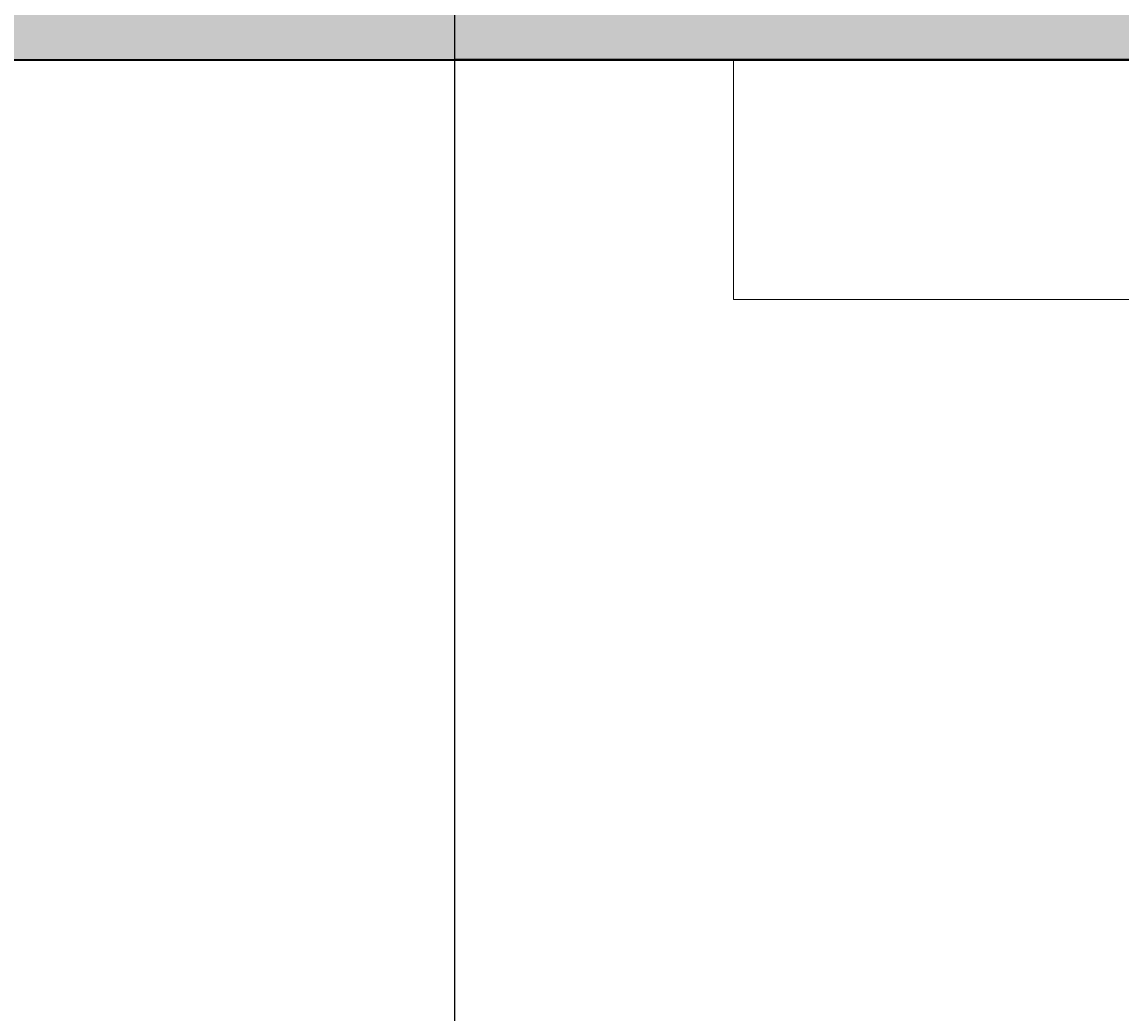
# Model space of a CAD drawing. Units: inches. Extents: x 1998 to 2588, y 1139 to 1977.
# Tile 84 of 134: x 2397 to 2425, y 1452 to 1477. Entities that reach past the tile are written whole.
import ezdxf

# ---------------------------------------------------------------- set-up
doc = ezdxf.new("R2010")
doc.units = ezdxf.units.IN
for name, color, linetype, lineweight in [('A-ANNO-DIMS', 2, 'Continuous', 18), ('A-WALL-PATT', 252, 'Continuous', 13), ('FUR', 21, 'Continuous', 18), ('WALL', 200, 'Continuous', 35)]:
    doc.layers.add(name, color=color, linetype=linetype, lineweight=lineweight)
doc.styles.get("Standard").update_dxf_attribs({"font": 'arial.ttf'})
doc.dimstyles.get("Standard").update_dxf_attribs({"dimtxt": 0.18, "dimasz": 0.18, "dimexe": 0.18, "dimexo": 0.0625, "dimgap": 0.09, "dimtad": 0, "dimtih": 1, "dimtoh": 1, "dimdec": 4, "dimzin": 0, "dimdsep": 46, "dimtxsty": 'Standard', "dimcen": 0.09, "dimadec": 0, "dimazin": 0, "dimtfac": 1, "dimtdec": 4, "dimtofl": 0, "dimtmove": 0, "dimatfit": 3, "dimfxl": 1, "dimtolj": 1, "dimtzin": 0, "dimarcsym": 0})

# ---------------------------------------------------------------- blocks, each defined once
blk = doc.blocks.new('CONSOLE-WALL')
blk.add_lwpolyline([(0, 6.123), (71.98, 6.123), (71.98, 0), (0, 0)], close=True)
blk = doc.blocks.new('*D23')
at = {"layer": 'A-ANNO-DIMS', "color": 0, "lineweight": -2, "transparency": 16777216}
for p, q in [((2549.179, 1476.17), (2549.179, 1138.602)), ((2059.473, 1413.17), (2059.473, 1138.602)), ((2059.653, 1138.782), (2303.928, 1138.782)), ((2548.999, 1138.782), (2304.723, 1138.782))]:
    blk.add_line(p, q, dxfattribs=at)
at = {"layer": 'A-ANNO-DIMS', "color": 0, "transparency": 16777216}
for points in [[(2059.653, 1138.812), (2059.653, 1138.752), (2059.473, 1138.782)], [(2548.999, 1138.812), (2548.999, 1138.752), (2549.179, 1138.782)]]:
    blk.add_solid(points, dxfattribs=at)
at = {"layer": 'Defpoints', "color": 0, "transparency": 16777216}
for p in [(2549.179, 1476.232), (2059.473, 1413.232), (2549.179, 1138.782)]:
    blk.add_point(p, dxfattribs=at)
at = {"layer": 'A-ANNO-DIMS', "color": 0, "transparency": 16777216, "insert": (2304.326, 1138.782), "char_height": 0.18, "attachment_point": 5}
blk.add_mtext('\\A1;489.7', dxfattribs=at)
blk = doc.blocks.new('*D24')
at = {"layer": 'A-ANNO-DIMS', "color": 0, "lineweight": -2, "transparency": 16777216}
for p, q in [((2398.535, 1911.232), (2588.309, 1911.232)), ((2588.129, 1911.052), (2588.129, 1570.164)), ((2588.129, 1228.912), (2588.129, 1569.8)), ((2527.535, 1228.732), (2588.309, 1228.732))]:
    blk.add_line(p, q, dxfattribs=at)
at = {"layer": 'A-ANNO-DIMS', "color": 0, "transparency": 16777216}
for points in [[(2588.099, 1911.052), (2588.159, 1911.052), (2588.129, 1911.232)], [(2588.099, 1228.912), (2588.159, 1228.912), (2588.129, 1228.732)]]:
    blk.add_solid(points, dxfattribs=at)
at = {"layer": 'Defpoints', "color": 0, "transparency": 16777216}
for p in [(2398.473, 1911.232), (2588.129, 1911.232), (2527.473, 1228.732)]:
    blk.add_point(p, dxfattribs=at)
at = {"layer": 'A-ANNO-DIMS', "color": 0, "transparency": 16777216, "insert": (2588.129, 1569.982), "char_height": 0.18, "attachment_point": 5}
blk.add_mtext('\\A1;682.5', dxfattribs=at)
blk = doc.blocks.new('*D33')
at = {"layer": 'A-ANNO-DIMS', "color": 0, "lineweight": -2, "transparency": 16777216}
for p, q in [((2407.973, 1480.67), (2407.973, 1138.602)), ((2498.179, 1480.67), (2498.179, 1138.602)), ((2408.153, 1138.782), (2452.753, 1138.782)), ((2497.999, 1138.782), (2453.399, 1138.782))]:
    blk.add_line(p, q, dxfattribs=at)
at = {"layer": 'A-ANNO-DIMS', "color": 0, "transparency": 16777216}
for points in [[(2408.153, 1138.812), (2408.153, 1138.752), (2407.973, 1138.782)], [(2497.999, 1138.812), (2497.999, 1138.752), (2498.179, 1138.782)]]:
    blk.add_solid(points, dxfattribs=at)
at = {"layer": 'Defpoints', "color": 0, "transparency": 16777216}
for p in [(2407.973, 1480.732), (2498.179, 1480.732), (2498.179, 1138.782)]:
    blk.add_point(p, dxfattribs=at)
at = {"layer": 'A-ANNO-DIMS', "color": 0, "transparency": 16777216, "insert": (2453.076, 1138.782), "char_height": 0.18, "attachment_point": 5}
blk.add_mtext('\\A1;90.2', dxfattribs=at)
blk = doc.blocks.new('*D43')
at = {"layer": 'A-ANNO-DIMS', "color": 0, "lineweight": -2, "transparency": 16777216}
for p, q in [((2407.973, 1594.67), (2407.973, 1138.602)), ((2345.973, 1588.67), (2345.973, 1138.602)), ((2346.153, 1138.782), (2376.754, 1138.782)), ((2407.793, 1138.782), (2377.191, 1138.782))]:
    blk.add_line(p, q, dxfattribs=at)
at = {"layer": 'A-ANNO-DIMS', "color": 0, "transparency": 16777216}
for points in [[(2346.153, 1138.812), (2346.153, 1138.752), (2345.973, 1138.782)], [(2407.793, 1138.812), (2407.793, 1138.752), (2407.973, 1138.782)]]:
    blk.add_solid(points, dxfattribs=at)
at = {"layer": 'Defpoints', "color": 0, "transparency": 16777216}
for p in [(2407.973, 1594.732), (2345.973, 1588.732), (2407.973, 1138.782)]:
    blk.add_point(p, dxfattribs=at)
at = {"layer": 'A-ANNO-DIMS', "color": 0, "transparency": 16777216, "insert": (2376.973, 1138.782), "char_height": 0.18, "attachment_point": 5}
blk.add_mtext('\\A1;62', dxfattribs=at)

msp = doc.modelspace()

# ---------------------------------------------------------------- hatches: boundary and pattern name
at = {"layer": 'A-WALL-PATT'}
h = msp.add_hatch(color=256, dxfattribs=at)
h.dxf.hatch_style = 1
h.paths.add_polyline_path([(2527.4729, 1362.2324), (2510.9729, 1362.2324), (2510.9729, 1357.7324), (2518.4729, 1357.7324), (2518.4729, 1237.7324), (2503.1458, 1237.7324), (2503.1458, 1228.7324), (2527.4729, 1228.7324)])
h.paths.add_polyline_path([(2490.5682, 1362.2324), (2398.4729, 1362.2324), (2398.4729, 1357.7324), (2490.5682, 1357.7324)])
h.paths.add_polyline_path([(2224.9729, 1264.7324), (2222.9729, 1264.7324), (2222.9729, 1232.4125), (2341.4729, 1232.4125), (2341.4729, 1234.4125), (2224.9729, 1234.4125)])
h.paths.add_polyline_path([(2334.5332, 1273.7324), (2264.7638, 1273.7324), (2264.7638, 1269.5611, -0.043659), (2264.3413, 1264.7324), (2334.5332, 1264.7324)])
h.paths.add_polyline_path([(2236.9551, 1273.7324), (2234.4125, 1273.7324), (2234.4125, 1264.7324), (2236.9551, 1264.7324), (2236.9551, 1269.5611)])
h.paths.add_polyline_path([(2222.9729, 1293.2324), (2096.9729, 1293.2324), (2096.9729, 1345.0966), (2087.9729, 1345.0966), (2087.9729, 1284.2324), (2222.9729, 1284.2324), (2222.9729, 1285.137)])
h.paths.add_polyline_path([(2096.9729, 1458.7927), (2087.9729, 1458.7927), (2087.9729, 1417.7324), (2087.9729, 1413.2324), (2096.9729, 1413.2324), (2096.9729, 1417.7324)])
h.paths.add_polyline_path([(2096.9729, 1413.2324), (2087.9729, 1413.2324), (2087.9729, 1365.5012), (2096.9729, 1365.5012), (2096.9729, 1369.3358)])
h.paths.add_polyline_path([(2186.2943, 1417.7324), (2138.6074, 1417.7324), (2096.9729, 1417.7324), (2096.9729, 1413.2324), (2138.6074, 1413.2324), (2186.2943, 1413.2324)])
h.paths.add_polyline_path([(2181.4729, 1465.7324), (2176.9729, 1465.7324), (2176.9729, 1451.6434), (2181.4729, 1451.6434)])
h.paths.add_polyline_path([(2181.4729, 1422.1664), (2176.9729, 1422.1664), (2176.9729, 1417.7324), (2181.4729, 1417.7324)])
h.paths.add_polyline_path([(2063.9729, 1465.7324), (2087.9729, 1465.7324), (2087.9729, 1470.2324), (2059.4729, 1470.2324), (2059.4729, 1413.2324), (2087.9729, 1413.2324), (2087.9729, 1417.7324), (2063.9729, 1417.7324)])
h.paths.add_polyline_path([(2181.4729, 1755.2324), (2176.9729, 1755.2324), (2176.9729, 1748.6798), (2177.0513, 1748.6798), (2181.4729, 1748.6798)])
h.paths.add_polyline_path([(2227.4729, 1707.2324), (2220.4647, 1707.2324), (2220.4647, 1702.7324), (2222.9729, 1702.7324), (2222.9729, 1604.637), (2227.4729, 1604.637)])
h.paths.add_polyline_path([(2114.9729, 1702.7324), (2105.9729, 1702.7324), (2105.9729, 1628.4781, -0.0318759), (2110.1012, 1628.7416), (2114.9729, 1628.7416)])
h.paths.add_polyline_path([(2345.9729, 1739.3278), (2341.4729, 1739.3278), (2341.4729, 1647.5211), (2345.9729, 1647.5211)])
h.paths.add_polyline_path([(2350.6273, 1641.2324), (2345.9729, 1641.2324), (2345.9729, 1636.7324), (2350.6273, 1636.7324), (2350.6273, 1639.8729)])
h.paths.add_polyline_path([(2501.9729, 1641.2324), (2407.9729, 1641.2324), (2392.5005, 1641.2324), (2392.5005, 1639.8729), (2392.5005, 1636.7324), (2501.9729, 1636.7324)])
h.paths.add_polyline_path([(2510.9729, 1755.2324), (2501.9729, 1755.2324), (2501.9729, 1641.2324), (2510.9729, 1641.2324)])
h.paths.add_polyline_path([(2549.1786, 1641.2324), (2522.3775, 1641.2324), (2522.3775, 1636.7324), (2540.1786, 1636.7324), (2540.1786, 1480.7324), (2522.3775, 1480.7324), (2522.3775, 1476.2324), (2549.1786, 1476.2324)])
h.paths.add_polyline_path([(2498.1786, 1594.7324), (2407.9729, 1594.7324), (2407.9729, 1585.7324), (2416.9729, 1585.7324), (2489.1786, 1585.7324), (2489.1786, 1531.7324), (2416.9729, 1531.7324), (2407.9729, 1531.7324), (2407.9729, 1522.7324), (2498.1786, 1522.7324)])
h.paths.add_polyline_path([(2351.6437, 1480.7324), (2345.9729, 1480.7324), (2345.9729, 1476.2324), (2351.6437, 1476.2324), (2351.6437, 1477.5919)])
h.paths.add_polyline_path([(2501.9729, 1480.7324), (2498.1786, 1480.7324), (2407.9729, 1480.7324), (2393.5168, 1480.7324), (2393.5168, 1477.5919), (2393.5168, 1476.2324), (2501.9729, 1476.2324)])

# ---------------------------------------------------------------- linework, layer by layer
at = {"layer": 'WALL'}
for p, q in [((2392.6008, 1476.2324), (2407.9729, 1476.2324)), ((2392.6008, 1476.2324), (2501.9729, 1476.2324)), ((2501.9729, 1476.2324), (2407.9729, 1476.2324))]:
    msp.add_line(p, q, dxfattribs=at)

# ---------------------------------------------------------------- block references
at = {"layer": 'FUR'}
msp.add_blockref('CONSOLE-WALL', (2415.1012, 1470.109), dxfattribs=at)

# ---------------------------------------------------------------- dimensions: what is measured, and where the dimension line sits
at = {"layer": 'A-ANNO-DIMS'}
dim = msp.add_linear_dim(base=(2588.1286, 1911.2324), p1=(2527.4729, 1228.7324), p2=(2398.4729, 1911.2324), angle=90, dimstyle='Standard', override={"dimdec": 1, "dimlfac": 1, "dimrnd": 0, "dimzin": 0, "dimdsep": 46, "dimlunit": 2}, dxfattribs=at)
dim.commit()
dim.dimension.update_dxf_attribs({"geometry": '*D24', "text_midpoint": (2588.1286, 1569.9824)})
for base, p1, p2, override, picture, middle in [((2407.9729, 1138.7824), (2345.9729, 1588.7324), (2407.9729, 1594.7324), {"dimdec": 0, "dimlfac": 1, "dimrnd": 0, "dimzin": 0, "dimdsep": 46, "dimlunit": 2}, '*D43', (2376.9729, 1138.7824)), ((2498.1786, 1138.7824), (2407.9729, 1480.7324), (2498.1786, 1480.7324), {"dimdec": 1, "dimlfac": 1, "dimrnd": 0, "dimzin": 0, "dimdsep": 46, "dimlunit": 2}, '*D33', (2453.0757, 1138.7824)), ((2549.1786, 1138.7824), (2059.4729, 1413.2324), (2549.1786, 1476.2324), {"dimdec": 1, "dimlfac": 1, "dimrnd": 0, "dimzin": 0, "dimdsep": 46, "dimlunit": 2}, '*D23', (2304.3257, 1138.7824))]:
    dim = msp.add_linear_dim(base=base, p1=p1, p2=p2, dimstyle='Standard', override=override, dxfattribs=at)
    dim.commit()
    dim.dimension.update_dxf_attribs({"geometry": picture, "text_midpoint": middle})

doc.saveas('drawing.dxf')
